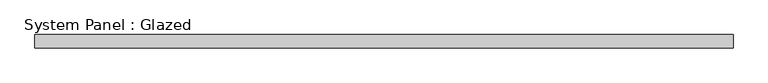
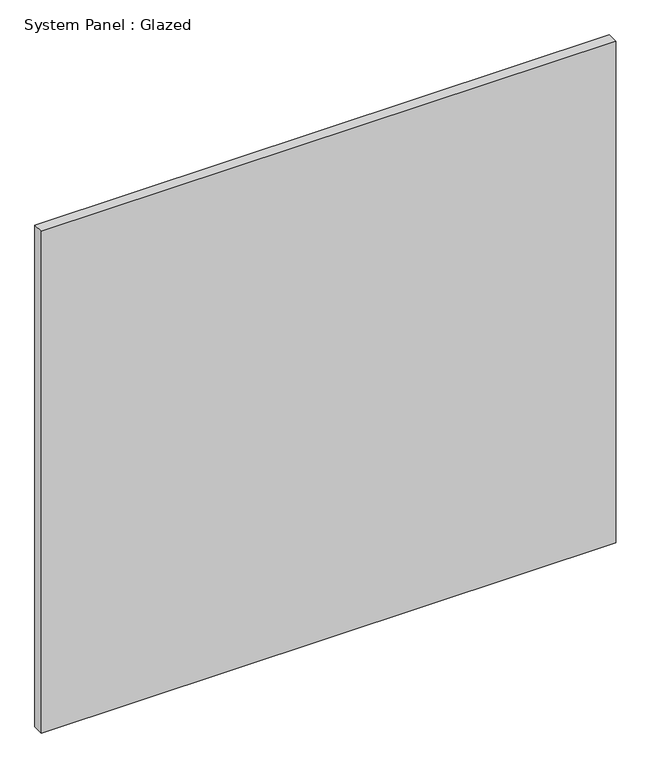
"""IFC4 building model written with IfcOpenShell, lengths in millimetres: plate geometry, System Panel : Glazed."""

from ifc_helpers import new_model, si_unit, origin, origin_with_axes, place, context, project, spatial, polyline, outline, extrude, source, transform, mapped, element, save


def system_panel_glazed_a9b6887b(model_context):
    return source(origin(), model_context, "Body", "SweptSolid", [
        extrude(outline(polyline([(660.4, 19.05), (-660.4, 19.05), (-660.4, 44.45), (660.4, 44.45), (660.4, 19.05)])), origin_with_axes(), (0.0, 0.0, 1.0), 1219.2),
    ])


if __name__ == "__main__":
    model = new_model("IFC4")
    model_context = context("Model", 3, world=origin())
    ifc_project = project(units=[si_unit("LENGTHUNIT", "METRE", prefix="MILLI")], contexts=[model_context])
    site = spatial("IfcSite", under=ifc_project)
    building = spatial("IfcBuilding", under=site)
    placement = place(None, origin())
    system_panel_glazed_shape = system_panel_glazed_a9b6887b(model_context)
    element("IfcPlate", 1, ObjectType="System Panel : Glazed", at=placement, inside=building, context=model_context, shape_type="MappedRepresentation", body=[
        mapped(system_panel_glazed_shape, transform((0.0, 0.0, 0.0), x_axis=(1.0, 0.0, 0.0), y_axis=(0.0, 1.0, 0.0), z_axis=(0.0, 0.0, 1.0))),
    ])
    save(model, "model.ifc")

# Revit data of these elements
# Type "System Panel : Glazed"
#   Construction Type Id = "GSP4R"
#   Analytic Construction = "1/8 in Pilkington single glazing"
#   Visual Light Transmittance = 0.9
#   Solar Heat Gain Coefficient = 0.86
#   Heat Transfer Coefficient (U) = 1.18115 BTU/(h·ft²·°F)
# Element 1 (IfcPlate, "System Panel : Glazed")
#   Materials on its faces: "Glass"
# Materials
#   "Glass": class "Glass", colour RGB 0 128 192, transparency 0.75, Description = "Soda Lime Glass", Cost = 0
